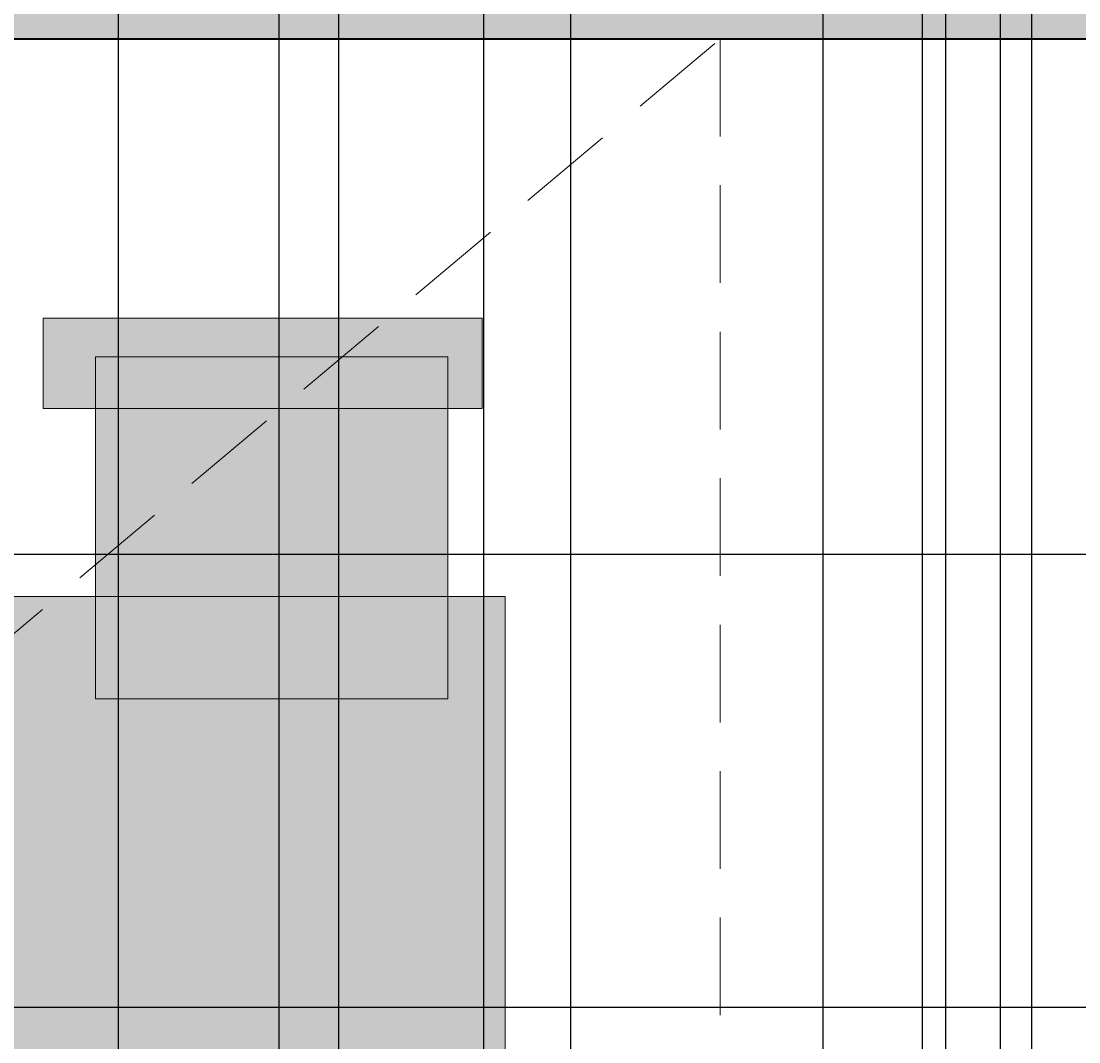
# Model space of a CAD drawing. Units: inches. Extents: x 818 to 1898, y 976 to 2364.
# Tile 76 of 96: x 1372 to 1439, y 1980 to 2045. Entities that reach past the tile are written whole.
import ezdxf

# ---------------------------------------------------------------- set-up
doc = ezdxf.new("R2010")
doc.units = ezdxf.units.IN
doc.header["$LTSCALE"] = 5
doc.header["$MEASUREMENT"] = 0
doc.linetypes.add('HIDDEN', pattern=[0.375, 0.25, -0.125])
for name, color, linetype, lineweight in [('A-ANNO-DIMS', 2, 'Continuous', 18), ('A-FLOR-OVHD', 8, 'HIDDEN', 13), ('A-FURN', 8, 'Continuous', 18), ('A-FURN-PATT', 8, 'Continuous', 9), ('A-GLAZ', 4, 'Continuous', 18), ('A-WALL', 7, 'Continuous', 40)]:
    doc.layers.add(name, color=color, linetype=linetype, lineweight=lineweight)
doc.layers.add('A-GLAZ-PATT', color=141, linetype='Continuous', lineweight=9, true_color=0xadddf7)
doc.layers.add('A-WALL-PATT', color=251, linetype='Continuous', lineweight=13, true_color=0x636466)
doc.styles.get("Standard").update_dxf_attribs({"font": 'arial.ttf'})
doc.dimstyles.get("Standard").update_dxf_attribs({"dimtxt": 0.18, "dimasz": 0.18, "dimexe": 0.18, "dimexo": 0.0625, "dimgap": 0.09, "dimtad": 0, "dimtih": 1, "dimtoh": 1, "dimdec": 4, "dimzin": 0, "dimdsep": 46, "dimtxsty": 'Standard', "dimcen": 0.09, "dimadec": 0, "dimazin": 0, "dimtfac": 1, "dimtdec": 4, "dimtofl": 0, "dimtmove": 0, "dimatfit": 3, "dimfxl": 1, "dimtolj": 1, "dimtzin": 0, "dimarcsym": 0})

# ---------------------------------------------------------------- blocks, each defined once
blk = doc.blocks.new('*D61')
at = {"layer": 'A-ANNO-DIMS', "color": 0, "lineweight": -2, "ltscale": 5, "transparency": 16777216}
for p, q in [((1071.725, 1203.027), (1071.725, 2363.873)), ((1071.905, 2363.693), (1250.936, 2363.693)), ((1430.545, 2363.693), (1251.514, 2363.693)), ((1430.725, 1203.027), (1430.725, 2363.873))]:
    blk.add_line(p, q, dxfattribs=at)
at = {"layer": 'A-ANNO-DIMS', "color": 0, "ltscale": 5, "transparency": 16777216}
for points in [[(1071.905, 2363.723), (1071.905, 2363.663), (1071.725, 2363.693)], [(1430.545, 2363.723), (1430.545, 2363.663), (1430.725, 2363.693)]]:
    blk.add_solid(points, dxfattribs=at)
at = {"layer": 'Defpoints', "color": 0, "ltscale": 5, "transparency": 16777216}
for p in [(1430.725, 2363.693), (1071.725, 1202.964), (1430.725, 1202.964)]:
    blk.add_point(p, dxfattribs=at)
at = {"layer": 'A-ANNO-DIMS', "color": 0, "ltscale": 5, "transparency": 16777216, "insert": (1251.225, 2363.693), "char_height": 0.18, "attachment_point": 5}
blk.add_mtext('\\A1;359', dxfattribs=at)
blk = doc.blocks.new('*D64')
at = {"layer": 'A-ANNO-DIMS', "color": 0, "lineweight": -2, "ltscale": 5, "transparency": 16777216}
for p, q in [((1197.725, 1501.141), (1197.725, 2363.873)), ((1197.905, 2363.693), (1313.935, 2363.693)), ((1430.545, 2363.693), (1314.516, 2363.693)), ((1430.725, 1501.141), (1430.725, 2363.873))]:
    blk.add_line(p, q, dxfattribs=at)
at = {"layer": 'A-ANNO-DIMS', "color": 0, "ltscale": 5, "transparency": 16777216}
for points in [[(1197.905, 2363.723), (1197.905, 2363.663), (1197.725, 2363.693)], [(1430.545, 2363.723), (1430.545, 2363.663), (1430.725, 2363.693)]]:
    blk.add_solid(points, dxfattribs=at)
at = {"layer": 'Defpoints', "color": 0, "ltscale": 5, "transparency": 16777216}
for p in [(1430.725, 2363.693), (1197.725, 1501.078), (1430.725, 1501.078)]:
    blk.add_point(p, dxfattribs=at)
at = {"layer": 'A-ANNO-DIMS', "color": 0, "ltscale": 5, "transparency": 16777216, "insert": (1314.225, 2363.693), "char_height": 0.18, "attachment_point": 5}
blk.add_mtext('\\A1;233', dxfattribs=at)
blk = doc.blocks.new('*D73')
at = {"layer": 'A-ANNO-DIMS', "color": 0, "lineweight": -2, "ltscale": 5, "transparency": 16777216}
for p, q in [((1590.663, 2011.078), (818.026, 2011.078)), ((818.206, 2010.898), (818.206, 1996.76)), ((818.206, 1982.258), (818.206, 1996.396)), ((1590.663, 1982.078), (818.026, 1982.078))]:
    blk.add_line(p, q, dxfattribs=at)
at = {"layer": 'A-ANNO-DIMS', "color": 0, "ltscale": 5, "transparency": 16777216}
for points in [[(818.176, 2010.898), (818.236, 2010.898), (818.206, 2011.078)], [(818.176, 1982.258), (818.236, 1982.258), (818.206, 1982.078)]]:
    blk.add_solid(points, dxfattribs=at)
at = {"layer": 'Defpoints', "color": 0, "ltscale": 5, "transparency": 16777216}
for p in [(818.206, 2011.078), (1590.725, 2011.078), (1590.725, 1982.078)]:
    blk.add_point(p, dxfattribs=at)
at = {"layer": 'A-ANNO-DIMS', "color": 0, "ltscale": 5, "transparency": 16777216, "insert": (818.206, 1996.578), "char_height": 0.18, "attachment_point": 5}
blk.add_mtext('\\A1;29', dxfattribs=at)
blk = doc.blocks.new('*D85')
at = {"layer": 'A-ANNO-DIMS', "color": 0, "lineweight": -2, "ltscale": 5, "transparency": 16777216}
for p, q in [((1258.788, 2053.078), (1897.916, 2053.078)), ((1897.736, 2052.898), (1897.736, 1876.76)), ((1897.736, 1700.258), (1897.736, 1876.396)), ((1258.788, 1700.078), (1897.916, 1700.078))]:
    blk.add_line(p, q, dxfattribs=at)
at = {"layer": 'A-ANNO-DIMS', "color": 0, "ltscale": 5, "transparency": 16777216}
for points in [[(1897.706, 2052.898), (1897.766, 2052.898), (1897.736, 2053.078)], [(1897.706, 1700.258), (1897.766, 1700.258), (1897.736, 1700.078)]]:
    blk.add_solid(points, dxfattribs=at)
at = {"layer": 'Defpoints', "color": 0, "ltscale": 5, "transparency": 16777216}
for p in [(1258.725, 2053.078), (1897.736, 2053.078), (1258.725, 1700.078)]:
    blk.add_point(p, dxfattribs=at)
at = {"layer": 'A-ANNO-DIMS', "color": 0, "ltscale": 5, "transparency": 16777216, "insert": (1897.736, 1876.578), "char_height": 0.18, "attachment_point": 5}
blk.add_mtext('\\A1;353', dxfattribs=at)
blk = doc.blocks.new('*D98')
at = {"layer": 'A-ANNO-DIMS', "color": 0, "lineweight": -2, "ltscale": 5, "transparency": 16777216}
for p, q in [((1338.541, 1071.118), (1338.541, 2363.873)), ((1338.721, 2363.693), (1364.815, 2363.693)), ((1391.696, 2363.693), (1365.602, 2363.693)), ((1391.876, 1071.118), (1391.876, 2363.873))]:
    blk.add_line(p, q, dxfattribs=at)
at = {"layer": 'A-ANNO-DIMS', "color": 0, "ltscale": 5, "transparency": 16777216}
for points in [[(1338.721, 2363.723), (1338.721, 2363.663), (1338.541, 2363.693)], [(1391.696, 2363.723), (1391.696, 2363.663), (1391.876, 2363.693)]]:
    blk.add_solid(points, dxfattribs=at)
at = {"layer": 'Defpoints', "color": 0, "ltscale": 5, "transparency": 16777216}
for p in [(1391.876, 2363.693), (1338.541, 1071.055), (1391.876, 1071.055)]:
    blk.add_point(p, dxfattribs=at)
at = {"layer": 'A-ANNO-DIMS', "color": 0, "ltscale": 5, "transparency": 16777216, "insert": (1365.208, 2363.693), "char_height": 0.18, "attachment_point": 5}
blk.add_mtext('\\A1;53.33', dxfattribs=at)
blk = doc.blocks.new('*D99')
at = {"layer": 'A-ANNO-DIMS', "color": 0, "lineweight": -2, "ltscale": 5, "transparency": 16777216}
for p, q in [((1391.876, 1071.118), (1391.876, 2363.873)), ((1392.056, 2363.693), (1420.454, 2363.693)), ((1449.64, 2363.693), (1421.241, 2363.693)), ((1449.82, 1071.118), (1449.82, 2363.873))]:
    blk.add_line(p, q, dxfattribs=at)
at = {"layer": 'A-ANNO-DIMS', "color": 0, "ltscale": 5, "transparency": 16777216}
for points in [[(1392.056, 2363.723), (1392.056, 2363.663), (1391.876, 2363.693)], [(1449.64, 2363.723), (1449.64, 2363.663), (1449.82, 2363.693)]]:
    blk.add_solid(points, dxfattribs=at)
at = {"layer": 'Defpoints', "color": 0, "ltscale": 5, "transparency": 16777216}
for p in [(1449.82, 2363.693), (1391.876, 1071.055), (1449.82, 1071.055)]:
    blk.add_point(p, dxfattribs=at)
at = {"layer": 'A-ANNO-DIMS', "color": 0, "ltscale": 5, "transparency": 16777216, "insert": (1420.848, 2363.693), "char_height": 0.18, "attachment_point": 5}
blk.add_mtext('\\A1;57.94', dxfattribs=at)
blk = doc.blocks.new('*D161')
at = {"layer": 'A-ANNO-DIMS', "color": 0, "lineweight": -2, "ltscale": 5, "transparency": 16777216}
for p, q in [((1429.225, 1876.141), (1429.225, 2363.873)), ((1429.405, 2363.693), (1509.589, 2363.693)), ((1590.545, 2363.693), (1510.361, 2363.693)), ((1590.725, 1876.141), (1590.725, 2363.873))]:
    blk.add_line(p, q, dxfattribs=at)
at = {"layer": 'A-ANNO-DIMS', "color": 0, "ltscale": 5, "transparency": 16777216}
for points in [[(1429.405, 2363.723), (1429.405, 2363.663), (1429.225, 2363.693)], [(1590.545, 2363.723), (1590.545, 2363.663), (1590.725, 2363.693)]]:
    blk.add_solid(points, dxfattribs=at)
at = {"layer": 'Defpoints', "color": 0, "ltscale": 5, "transparency": 16777216}
for p in [(1590.725, 2363.693), (1429.225, 1876.078), (1590.725, 1876.078)]:
    blk.add_point(p, dxfattribs=at)
at = {"layer": 'A-ANNO-DIMS', "color": 0, "ltscale": 5, "transparency": 16777216, "insert": (1509.975, 2363.693), "char_height": 0.18, "attachment_point": 5}
blk.add_mtext('\\A1;161.5', dxfattribs=at)
blk = doc.blocks.new('*D166')
at = {"layer": 'A-ANNO-DIMS', "color": 0, "lineweight": -2, "ltscale": 5, "transparency": 16777216}
for p, q in [((1401.146, 1510.141), (1401.146, 2363.873)), ((1401.326, 2363.693), (1415.54, 2363.693)), ((1430.545, 2363.693), (1416.331, 2363.693)), ((1430.725, 1510.141), (1430.725, 2363.873))]:
    blk.add_line(p, q, dxfattribs=at)
at = {"layer": 'A-ANNO-DIMS', "color": 0, "ltscale": 5, "transparency": 16777216}
for points in [[(1401.326, 2363.723), (1401.326, 2363.663), (1401.146, 2363.693)], [(1430.545, 2363.723), (1430.545, 2363.663), (1430.725, 2363.693)]]:
    blk.add_solid(points, dxfattribs=at)
at = {"layer": 'Defpoints', "color": 0, "ltscale": 5, "transparency": 16777216}
for p in [(1430.725, 2363.693), (1401.146, 1510.078), (1430.725, 1510.078)]:
    blk.add_point(p, dxfattribs=at)
at = {"layer": 'A-ANNO-DIMS', "color": 0, "ltscale": 5, "transparency": 16777216, "insert": (1415.936, 2363.693), "char_height": 0.18, "attachment_point": 5}
blk.add_mtext('\\A1;29.58', dxfattribs=at)
blk = doc.blocks.new('*D191')
at = {"layer": 'A-ANNO-DIMS', "color": 0, "lineweight": -2, "ltscale": 5, "transparency": 16777216}
for p, q in [((1434.225, 1409.115), (1434.225, 2363.873)), ((1434.405, 2363.693), (1435.076, 2363.693)), ((1436.045, 2363.693), (1435.375, 2363.693)), ((1436.225, 1409.115), (1436.225, 2363.873))]:
    blk.add_line(p, q, dxfattribs=at)
at = {"layer": 'A-ANNO-DIMS', "color": 0, "ltscale": 5, "transparency": 16777216}
for points in [[(1434.405, 2363.723), (1434.405, 2363.663), (1434.225, 2363.693)], [(1436.045, 2363.723), (1436.045, 2363.663), (1436.225, 2363.693)]]:
    blk.add_solid(points, dxfattribs=at)
at = {"layer": 'Defpoints', "color": 0, "ltscale": 5, "transparency": 16777216}
for p in [(1436.225, 2363.693), (1434.225, 1409.052), (1436.225, 1409.052)]:
    blk.add_point(p, dxfattribs=at)
at = {"layer": 'A-ANNO-DIMS', "color": 0, "ltscale": 5, "transparency": 16777216, "insert": (1435.225, 2363.693), "char_height": 0.18, "attachment_point": 5}
blk.add_mtext('\\A1;2', dxfattribs=at)
blk = doc.blocks.new('*D207')
at = {"layer": 'A-ANNO-DIMS', "color": 0, "lineweight": -2, "ltscale": 5, "transparency": 16777216}
for p, q in [((1590.663, 2044.078), (818.026, 2044.078)), ((818.206, 2043.898), (818.206, 2027.76)), ((818.206, 2011.258), (818.206, 2027.396)), ((1590.663, 2011.078), (818.026, 2011.078))]:
    blk.add_line(p, q, dxfattribs=at)
at = {"layer": 'A-ANNO-DIMS', "color": 0, "ltscale": 5, "transparency": 16777216}
for points in [[(818.176, 2043.898), (818.236, 2043.898), (818.206, 2044.078)], [(818.176, 2011.258), (818.236, 2011.258), (818.206, 2011.078)]]:
    blk.add_solid(points, dxfattribs=at)
at = {"layer": 'Defpoints', "color": 0, "ltscale": 5, "transparency": 16777216}
for p in [(818.206, 2044.078), (1590.725, 2044.078), (1590.725, 2011.078)]:
    blk.add_point(p, dxfattribs=at)
at = {"layer": 'A-ANNO-DIMS', "color": 0, "ltscale": 5, "transparency": 16777216, "insert": (818.206, 2027.578), "char_height": 0.18, "attachment_point": 5}
blk.add_mtext('\\A1;33', dxfattribs=at)
blk = doc.blocks.new('*D252')
at = {"layer": 'A-ANNO-DIMS', "color": 0, "lineweight": -2, "ltscale": 5, "transparency": 16777216}
for p, q in [((1330.305, 2053.016), (1330.305, 975.663)), ((1388.031, 2053.016), (1388.031, 975.663)), ((1330.485, 975.843), (1358.775, 975.843)), ((1387.851, 975.843), (1359.562, 975.843))]:
    blk.add_line(p, q, dxfattribs=at)
at = {"layer": 'A-ANNO-DIMS', "color": 0, "ltscale": 5, "transparency": 16777216}
for points in [[(1330.485, 975.873), (1330.485, 975.813), (1330.305, 975.843)], [(1387.851, 975.873), (1387.851, 975.813), (1388.031, 975.843)]]:
    blk.add_solid(points, dxfattribs=at)
at = {"layer": 'Defpoints', "color": 0, "ltscale": 5, "transparency": 16777216}
for p in [(1330.305, 2053.078), (1388.031, 2053.078), (1388.031, 975.843)]:
    blk.add_point(p, dxfattribs=at)
at = {"layer": 'A-ANNO-DIMS', "color": 0, "ltscale": 5, "transparency": 16777216, "insert": (1359.168, 975.843), "char_height": 0.18, "attachment_point": 5}
blk.add_mtext('\\A1;57.73', dxfattribs=at)
blk = doc.blocks.new('*D273')
at = {"layer": 'A-ANNO-DIMS', "color": 0, "lineweight": -2, "ltscale": 5, "transparency": 16777216}
for p, q in [((1406.725, 1587.479), (1406.725, 2363.873)), ((1406.905, 2363.693), (1418.505, 2363.693)), ((1430.545, 2363.693), (1418.945, 2363.693)), ((1430.725, 1587.479), (1430.725, 2363.873))]:
    blk.add_line(p, q, dxfattribs=at)
at = {"layer": 'A-ANNO-DIMS', "color": 0, "ltscale": 5, "transparency": 16777216}
for points in [[(1406.905, 2363.723), (1406.905, 2363.663), (1406.725, 2363.693)], [(1430.545, 2363.723), (1430.545, 2363.663), (1430.725, 2363.693)]]:
    blk.add_solid(points, dxfattribs=at)
at = {"layer": 'Defpoints', "color": 0, "ltscale": 5, "transparency": 16777216}
for p in [(1430.725, 2363.693), (1406.725, 1587.416), (1430.725, 1587.416)]:
    blk.add_point(p, dxfattribs=at)
at = {"layer": 'A-ANNO-DIMS', "color": 0, "ltscale": 5, "transparency": 16777216, "insert": (1418.725, 2363.693), "char_height": 0.18, "attachment_point": 5}
blk.add_mtext('\\A1;24', dxfattribs=at)
blk = doc.blocks.new('*D274')
at = {"layer": 'A-ANNO-DIMS', "color": 0, "lineweight": -2, "ltscale": 5, "transparency": 16777216}
for p, q in [((1311.025, 1897.929), (1311.025, 2363.873)), ((1311.205, 2363.693), (1344.007, 2363.693)), ((1377.599, 2363.693), (1344.797, 2363.693)), ((1377.779, 1897.929), (1377.779, 2363.873))]:
    blk.add_line(p, q, dxfattribs=at)
at = {"layer": 'A-ANNO-DIMS', "color": 0, "ltscale": 5, "transparency": 16777216}
for points in [[(1311.205, 2363.723), (1311.205, 2363.663), (1311.025, 2363.693)], [(1377.599, 2363.723), (1377.599, 2363.663), (1377.779, 2363.693)]]:
    blk.add_solid(points, dxfattribs=at)
at = {"layer": 'Defpoints', "color": 0, "ltscale": 5, "transparency": 16777216}
for p in [(1377.779, 2363.693), (1311.025, 1897.866), (1377.779, 1897.866)]:
    blk.add_point(p, dxfattribs=at)
at = {"layer": 'A-ANNO-DIMS', "color": 0, "ltscale": 5, "transparency": 16777216, "insert": (1344.402, 2363.693), "char_height": 0.18, "attachment_point": 5}
blk.add_mtext('\\A1;66.75', dxfattribs=at)
blk = doc.blocks.new('*D281')
at = {"layer": 'A-ANNO-DIMS', "color": 0, "lineweight": -2, "ltscale": 5, "transparency": 16777216}
for p, q in [((1250.303, 1913.703), (1250.303, 2363.873)), ((1250.483, 2363.693), (1420.121, 2363.693)), ((1590.545, 2363.693), (1420.907, 2363.693)), ((1590.725, 2011.141), (1590.725, 2363.873))]:
    blk.add_line(p, q, dxfattribs=at)
at = {"layer": 'A-ANNO-DIMS', "color": 0, "ltscale": 5, "transparency": 16777216}
for points in [[(1250.483, 2363.723), (1250.483, 2363.663), (1250.303, 2363.693)], [(1590.545, 2363.723), (1590.545, 2363.663), (1590.725, 2363.693)]]:
    blk.add_solid(points, dxfattribs=at)
at = {"layer": 'Defpoints', "color": 0, "ltscale": 5, "transparency": 16777216}
for p in [(1590.725, 2363.693), (1590.725, 2011.078), (1250.303, 1913.64)]:
    blk.add_point(p, dxfattribs=at)
at = {"layer": 'A-ANNO-DIMS', "color": 0, "ltscale": 5, "transparency": 16777216, "insert": (1420.514, 2363.693), "char_height": 0.18, "attachment_point": 5}
blk.add_mtext('\\A1;340.4', dxfattribs=at)
blk = doc.blocks.new('*D282')
at = {"layer": 'A-ANNO-DIMS', "color": 0, "lineweight": -2, "ltscale": 5, "transparency": 16777216}
for p, q in [((1422.083, 2081.188), (1897.916, 2081.188)), ((1897.736, 2081.008), (1897.736, 1884.315)), ((1897.736, 1687.258), (1897.736, 1883.951)), ((1463.788, 1687.078), (1897.916, 1687.078))]:
    blk.add_line(p, q, dxfattribs=at)
at = {"layer": 'A-ANNO-DIMS', "color": 0, "ltscale": 5, "transparency": 16777216}
for points in [[(1897.706, 2081.008), (1897.766, 2081.008), (1897.736, 2081.188)], [(1897.706, 1687.258), (1897.766, 1687.258), (1897.736, 1687.078)]]:
    blk.add_solid(points, dxfattribs=at)
at = {"layer": 'Defpoints', "color": 0, "ltscale": 5, "transparency": 16777216}
for p in [(1422.02, 2081.188), (1897.736, 2081.188), (1463.725, 1687.078)]:
    blk.add_point(p, dxfattribs=at)
at = {"layer": 'A-ANNO-DIMS', "color": 0, "ltscale": 5, "transparency": 16777216, "insert": (1897.736, 1884.133), "char_height": 0.18, "attachment_point": 5}
blk.add_mtext('\\A1;394.1', dxfattribs=at)
blk = doc.blocks.new('*D288')
at = {"layer": 'A-ANNO-DIMS', "color": 0, "lineweight": -2, "ltscale": 5, "transparency": 16777216}
for p, q in [((1422.876, 1742.674), (1422.876, 2363.873)), ((1423.056, 2363.693), (1466.906, 2363.693)), ((1511.545, 2363.693), (1467.695, 2363.693)), ((1511.725, 1716.108), (1511.725, 2363.873))]:
    blk.add_line(p, q, dxfattribs=at)
at = {"layer": 'A-ANNO-DIMS', "color": 0, "ltscale": 5, "transparency": 16777216}
for points in [[(1423.056, 2363.723), (1423.056, 2363.663), (1422.876, 2363.693)], [(1511.545, 2363.723), (1511.545, 2363.663), (1511.725, 2363.693)]]:
    blk.add_solid(points, dxfattribs=at)
at = {"layer": 'Defpoints', "color": 0, "ltscale": 5, "transparency": 16777216}
for p in [(1511.725, 2363.693), (1422.876, 1742.611), (1511.725, 1716.045)]:
    blk.add_point(p, dxfattribs=at)
at = {"layer": 'A-ANNO-DIMS', "color": 0, "ltscale": 5, "transparency": 16777216, "insert": (1467.3, 2363.693), "char_height": 0.18, "attachment_point": 5}
blk.add_mtext('\\A1;88.85', dxfattribs=at)

msp = doc.modelspace()

# ---------------------------------------------------------------- hatches: boundary and pattern name
at = {"layer": 'A-FURN-PATT', "ltscale": 5}
h = msp.add_hatch(color=256, dxfattribs=at)
h.dxf.hatch_style = 1
h.paths.add_polyline_path([(1341.9997, 1981.5338), (1317.9034, 2001.8247), (1314.2595, 2001.8247), (1314.2595, 2004.893), (1310.1046, 2008.3917), (1303.9314, 2008.3917), (1303.9314, 1953.0408), (1308.1629, 1953.0408), (1314.2595, 1958.1746), (1314.2595, 1959.6079), (1315.9616, 1959.6079)])
h.paths.add_polyline_path([(1341.9997, 1981.5338), (1315.9616, 1959.6079), (1336.7936, 1959.6079), (1336.7936, 1953.0408), (1345.3966, 1953.0408), (1345.3966, 1959.6079), (1368.0379, 1959.6079)])
h.paths.add_polyline_path([(1402.518, 2008.3917), (1398.8475, 2008.3917), (1398.8475, 2001.8247), (1376.3134, 2001.8247), (1376.3134, 2008.3917), (1373.8948, 2008.3917), (1367.9307, 2003.3695), (1367.9307, 2001.8247), (1366.0961, 2001.8247), (1341.9997, 1981.5338), (1368.0379, 1959.6079), (1375.8366, 1953.0408), (1376.3134, 1953.0408), (1376.3134, 1959.6079), (1398.8475, 1959.6079), (1398.8475, 1953.0408), (1402.518, 1953.0408)])
h.paths.add_polyline_path([(1366.0961, 2001.8247), (1345.3966, 2001.8247), (1345.3966, 2008.3917), (1336.7936, 2008.3917), (1336.7936, 2001.8247), (1317.9034, 2001.8247), (1341.9997, 1981.5338)])
h.paths.add_polyline_path([(1336.7936, 1959.6079), (1315.9616, 1959.6079), (1314.2595, 1958.1746), (1314.2595, 1953.0408), (1336.7936, 1953.0408)], flags=17)
h.paths.add_polyline_path([(1367.9307, 1959.6079), (1345.3966, 1959.6079), (1345.3966, 1953.0408), (1367.9307, 1953.0408)], flags=17)
h.paths.add_polyline_path([(1398.8475, 1959.6079), (1376.3134, 1959.6079), (1376.3134, 1953.0408), (1398.8475, 1953.0408)], flags=17)
h.paths.add_polyline_path([(1368.0379, 1959.6079), (1367.9307, 1959.6079), (1367.9307, 1953.0408), (1375.8366, 1953.0408)], flags=17)
h.paths.add_polyline_path([(1314.2595, 1958.1746), (1308.1629, 1953.0408), (1314.2595, 1953.0408)], flags=17)
h.paths.add_polyline_path([(1315.9616, 1959.6079), (1314.2595, 1959.6079), (1314.2595, 1958.1746)], flags=16)
h.paths.add_polyline_path([(1314.2595, 2008.3917), (1310.1046, 2008.3917), (1314.2595, 2004.893)], flags=17)
h.paths.add_polyline_path([(1336.7936, 2008.3917), (1314.2595, 2008.3917), (1314.2595, 2004.893), (1317.9034, 2001.8247), (1336.7936, 2001.8247)], flags=17)
h.paths.add_polyline_path([(1314.2595, 2004.893), (1314.2595, 2001.8247), (1317.9034, 2001.8247)], flags=16)
h.paths.add_polyline_path([(1367.9307, 2008.3917), (1345.3966, 2008.3917), (1345.3966, 2001.8247), (1366.0961, 2001.8247), (1367.9307, 2003.3695)], flags=17)
h.paths.add_polyline_path([(1398.8475, 2008.3917), (1376.3134, 2008.3917), (1376.3134, 2001.8247), (1398.8475, 2001.8247)], flags=17)
h.paths.add_polyline_path([(1373.8948, 2008.3917), (1367.9307, 2008.3917), (1367.9307, 2003.3695)], flags=17)
h.paths.add_polyline_path([(1367.9307, 2003.3695), (1366.0961, 2001.8247), (1367.9307, 2001.8247)], flags=16)
h.paths.add_polyline_path([(1546.1595, 2044.0782), (1451.7698, 2044.0782), (1451.7698, 2020.0782), (1546.1595, 2020.0782)])
h.paths.add_polyline_path([(1492.0729, 2040.001, 0.431429), (1491.8238, 2040.251), (1491.3087, 2040.251, 0.415217), (1491.0729, 2040.001)], flags=16)
h.paths.add_polyline_path([(1481.8346, 2039.6036), (1511.886, 2039.6036), (1511.886, 2024.9917), (1481.8346, 2024.9917)], flags=16)
h.paths.add_polyline_path([(1491.0729, 2039.4857), (1491.0729, 2039.501), (1492.0729, 2039.501, -0.4117484), (1491.8401, 2039.251), (1491.8229, 2039.251), (1491.8229, 2039.2509, 0.4325918), (1492.0729, 2039.501), (1491.0729, 2039.501, 0.432604), (1491.3229, 2039.2509), (1491.3229, 2039.251), (1491.325, 2039.251, -0.4165823)], flags=0)
h.paths.add_polyline_path([(1485.3701, 2030.9622), (1485.3701, 2034.3556, -0.4142136), (1488.3701, 2037.3556), (1490.3421, 2037.3556, -0.0779193), (1491.0729, 2038.751), (1495.0729, 2038.751, -0.3148679), (1496.07, 2037.1201, -0.3016609), (1497.9049, 2034.3556), (1497.9049, 2030.9622, -0.4142136), (1494.9049, 2027.9622), (1488.3701, 2027.9622, -0.4142136)], flags=0)
h.paths.add_polyline_path([(1490.3229, 2035.751, 0.2655648), (1491.3229, 2036.751), (1491.3229, 2037.126), (1491.0729, 2037.126, -0.7914183), (1490.5434, 2037.251, -0.7914183), (1491.0729, 2037.376), (1491.3229, 2037.376), (1491.3229, 2037.751), (1492.0729, 2037.751), (1492.0729, 2037.376), (1492.3229, 2037.376, -0.7914183), (1492.8524, 2037.251, -0.7914183), (1492.3229, 2037.126), (1492.1491, 2037.126, -0.0866263), (1492.5376, 2036.0294, 0.1070481), (1493.0729, 2035.751), (1490.3229, 2035.751)], flags=0)
h.paths.add_polyline_path([(1491.9774, 2037.251, -1), (1491.4184, 2037.251, -1)], flags=0)
h.paths.add_polyline_path([(1500.0743, 2028.6045), (1500.0743, 2029.4074), (1510.8414, 2029.4074), (1510.8414, 2028.6045)], flags=0)
h.paths.add_polyline_path([(1500.0743, 2030.5314), (1500.0743, 2031.3342), (1510.8414, 2031.3342), (1510.8414, 2030.5314)], flags=0)
h.paths.add_polyline_path([(1500.0743, 2032.94), (1500.0743, 2033.7428), (1510.8414, 2033.7428), (1510.8414, 2032.94)], flags=0)
h.paths.add_polyline_path([(1500.0743, 2035.7499), (1500.0743, 2036.5528), (1510.8414, 2036.5528), (1510.8414, 2035.7499)], flags=0)
h.paths.add_polyline_path([(1590.7251, 2044.0782), (1576.1595, 2044.0782), (1576.1595, 2020.0782), (1590.7251, 2020.0782)])
h.paths.add_polyline_path([(1668.4429, 2044.0782), (1599.7252, 2044.0782), (1599.7252, 2020.0782), (1668.4429, 2020.0782)])
h.paths.add_polyline_path([(1621.2588, 2040.001, 0.431429), (1621.0097, 2040.251), (1620.4946, 2040.251, 0.415217), (1620.2588, 2040.001)], flags=16)
h.paths.add_polyline_path([(1611.0205, 2024.9917), (1611.0205, 2039.6036), (1641.0719, 2039.6036), (1641.0719, 2024.9917)], flags=16)
h.paths.add_polyline_path([(1620.2588, 2039.4857), (1620.2588, 2039.501), (1621.2588, 2039.501, -0.4117484), (1621.026, 2039.251), (1621.0088, 2039.251), (1621.0088, 2039.2509, 0.4325918), (1621.2588, 2039.501), (1620.2588, 2039.501, 0.432604), (1620.5088, 2039.2509), (1620.5088, 2039.251), (1620.5109, 2039.251, -0.4165823)], flags=0)
h.paths.add_polyline_path([(1614.556, 2030.9622), (1614.556, 2034.3556, -0.4142136), (1617.556, 2037.3556), (1619.528, 2037.3556, -0.0779193), (1620.2588, 2038.751), (1624.2588, 2038.751, -0.3148679), (1625.2559, 2037.1201, -0.3016609), (1627.0908, 2034.3556), (1627.0908, 2030.9622, -0.4142136), (1624.0908, 2027.9622), (1617.556, 2027.9622, -0.4142136)], flags=0)
h.paths.add_polyline_path([(1619.5088, 2035.751, 0.2655648), (1620.5088, 2036.751), (1620.5088, 2037.126), (1620.2588, 2037.126, -0.7914183), (1619.7293, 2037.251, -0.7914183), (1620.2588, 2037.376), (1620.5088, 2037.376), (1620.5088, 2037.751), (1621.2588, 2037.751), (1621.2588, 2037.376), (1621.5088, 2037.376, -0.7914183), (1622.0383, 2037.251, -0.7914183), (1621.5088, 2037.126), (1621.335, 2037.126, -0.0866263), (1621.7235, 2036.0294, 0.1070481), (1622.2588, 2035.751), (1619.5088, 2035.751)], flags=0)
h.paths.add_polyline_path([(1620.6043, 2037.251, -1), (1621.1633, 2037.251, -1)], flags=0)
h.paths.add_polyline_path([(1629.2602, 2028.6045), (1629.2602, 2029.4074), (1640.0273, 2029.4074), (1640.0273, 2028.6045)], flags=0)
h.paths.add_polyline_path([(1629.2602, 2030.5314), (1629.2602, 2031.3342), (1640.0273, 2031.3342), (1640.0273, 2030.5314)], flags=0)
h.paths.add_polyline_path([(1629.2602, 2032.94), (1629.2602, 2033.7428), (1640.0273, 2033.7428), (1640.0273, 2032.94)], flags=0)
h.paths.add_polyline_path([(1629.2602, 2035.7499), (1629.2602, 2036.5528), (1640.0273, 2036.5528), (1640.0273, 2035.7499)], flags=0)
h.paths.add_polyline_path([(1705.7252, 2044.0782), (1698.4429, 2044.0782), (1698.4429, 2020.0782), (1705.7252, 2020.0782)])
h.paths.add_polyline_path([(1705.7252, 1972.0782), (1599.7252, 1972.0782), (1599.7252, 1948.0782), (1705.7252, 1948.0782)])
h.paths.add_polyline_path([(1550.0109, 1979.2444), (1483.5451, 1979.2444), (1483.5451, 1948.6602), (1550.0109, 1948.6602)])
h.paths.add_polyline_path([(1490.2586, 1948.6602), (1488.2586, 1948.6602), (1488.2586, 1941.1742, 0.4142136), (1491.2586, 1938.1742), (1500.7446, 1938.1742, -0.4142136)])
h.paths.add_polyline_path([(1513.2306, 1941.1742), (1513.2306, 1948.6602), (1511.2306, 1948.6602, -0.4142136), (1500.7446, 1938.1742), (1510.2306, 1938.1742, 0.4142136)])
h.paths.add_polyline_path([(1518.778, 1948.6602), (1516.778, 1948.6602), (1516.778, 1941.1742, 0.4142136), (1519.778, 1938.1742), (1529.264, 1938.1742, -0.4142136)])
h.paths.add_polyline_path([(1541.75, 1941.1742), (1541.75, 1948.6602), (1539.75, 1948.6602, -0.4142136), (1529.264, 1938.1742), (1538.75, 1938.1742, 0.4142136)])
h.paths.add_polyline_path([(1590.7251, 1900.0782), (1519.6413, 1900.0782), (1519.6413, 1876.0782), (1590.7251, 1876.0782)])
h = msp.add_hatch(color=256, dxfattribs=at)
h.dxf.hatch_style = 1
h.paths.add_polyline_path([(1336.7936, 1953.0408), (1314.2595, 1953.0408), (1314.2595, 1941.0096), (1336.7936, 1941.0096)])
h.paths.add_polyline_path([(1338.9915, 1941.0096), (1336.7936, 1941.0096), (1336.7936, 1937.7177), (1314.2595, 1937.7177), (1314.2595, 1941.0096), (1310.9077, 1941.0096), (1310.9077, 1935.2252), (1338.9915, 1935.2252)])
h.paths.add_polyline_path([(1336.7936, 1941.0096), (1314.2595, 1941.0096), (1314.2595, 1937.7177), (1336.7936, 1937.7177)], flags=17)
h.paths.add_polyline_path([(1367.9307, 1959.6079), (1345.3966, 1959.6079), (1345.3966, 1941.0096), (1367.9307, 1941.0096)])
h.paths.add_polyline_path([(1398.8475, 1953.0408), (1376.3134, 1953.0408), (1376.3134, 1952.6393), (1390.1242, 1941.0096), (1398.8475, 1941.0096)])
h.paths.add_polyline_path([(1376.3134, 1952.6393), (1376.3134, 1941.0096), (1390.1242, 1941.0096)], flags=17)
h.paths.add_polyline_path([(1370.1286, 1941.0096), (1367.9307, 1941.0096), (1367.9307, 1937.7177), (1345.3966, 1937.7177), (1345.3966, 1941.0096), (1342.0448, 1941.0096), (1342.0448, 1935.2252), (1370.1286, 1935.2252)])
h.paths.add_polyline_path([(1367.9307, 1941.0096), (1345.3966, 1941.0096), (1345.3966, 1937.7177), (1367.9307, 1937.7177)], flags=17)
h.paths.add_polyline_path([(1390.1242, 1941.0096), (1376.3134, 1941.0096), (1376.3134, 1937.7177), (1394.0336, 1937.7177)], flags=17)
h.paths.add_polyline_path([(1394.0336, 1937.7177), (1376.3134, 1937.7177), (1376.3134, 1941.0096), (1372.9616, 1941.0096), (1372.9616, 1935.2252), (1396.9935, 1935.2252)])
h.paths.add_polyline_path([(1398.8475, 1941.0096), (1390.1242, 1941.0096), (1394.0336, 1937.7177), (1398.8475, 1937.7177)])
h.paths.add_polyline_path([(1401.0455, 1941.0096), (1398.8475, 1941.0096), (1398.8475, 1937.7177), (1394.0336, 1937.7177), (1396.9935, 1935.2252), (1401.0455, 1935.2252)])
h.paths.add_polyline_path([(1336.7936, 2020.4229), (1314.2595, 2020.4229), (1314.2595, 2008.3917), (1336.7936, 2008.3917)])
h.paths.add_polyline_path([(1336.7936, 2023.7149), (1314.2595, 2023.7149), (1314.2595, 2020.4229), (1336.7936, 2020.4229)], flags=17)
h.paths.add_polyline_path([(1338.9915, 2026.2074), (1310.9077, 2026.2074), (1310.9077, 2020.4229), (1314.2595, 2020.4229), (1314.2595, 2023.7149), (1336.7936, 2023.7149), (1336.7936, 2020.4229), (1338.9915, 2020.4229)])
h.paths.add_polyline_path([(1367.9307, 2023.7149), (1345.3966, 2023.7149), (1345.3966, 2020.4229), (1367.9307, 2020.4229)], flags=17)
h.paths.add_polyline_path([(1370.1286, 2026.2074), (1342.0448, 2026.2074), (1342.0448, 2020.4229), (1345.3966, 2020.4229), (1345.3966, 2023.7149), (1367.9307, 2023.7149), (1367.9307, 2020.4229), (1370.1286, 2020.4229)])
h.paths.add_polyline_path([(1367.9307, 2020.4229), (1345.3966, 2020.4229), (1345.3966, 2008.3917), (1367.9307, 2008.3917)])
h.paths.add_polyline_path([(1398.8475, 2020.4229), (1388.1824, 2020.4229), (1376.3134, 2010.4284), (1376.3134, 2008.3917), (1398.8475, 2008.3917)])
h.paths.add_polyline_path([(1392.0918, 2023.7149), (1376.3134, 2023.7149), (1376.3134, 2020.4229), (1388.1824, 2020.4229)], flags=17)
h.paths.add_polyline_path([(1388.1824, 2020.4229), (1376.3134, 2020.4229), (1376.3134, 2010.4284)], flags=17)
h.paths.add_polyline_path([(1395.0518, 2026.2074), (1372.9616, 2026.2074), (1372.9616, 2020.4229), (1376.3134, 2020.4229), (1376.3134, 2023.7149), (1392.0918, 2023.7149)])
h.paths.add_polyline_path([(1398.8475, 2023.7149), (1392.0918, 2023.7149), (1388.1824, 2020.4229), (1398.8475, 2020.4229)])
h.paths.add_polyline_path([(1401.0455, 2026.2074), (1395.0518, 2026.2074), (1392.0918, 2023.7149), (1398.8475, 2023.7149), (1398.8475, 2020.4229), (1401.0455, 2020.4229)])
h.paths.add_polyline_path([(1327.0339, 1897.8663), (1311.025, 1897.8663), (1311.025, 1876.0782), (1327.0339, 1876.0782)])
h.paths.add_polyline_path([(1377.7791, 1897.8663), (1359.9579, 1897.8663), (1359.9579, 1876.0782), (1377.7791, 1876.0782)])
h.paths.add_polyline_path([(1430.7251, 1541.0439), (1406.7251, 1541.0439), (1406.7251, 1525.9965), (1430.7251, 1525.9965)])
h.paths.add_polyline_path([(1430.7251, 1587.4164), (1406.7251, 1587.4164), (1406.7251, 1570.9187), (1430.7251, 1570.9187)])
at = {"layer": 'A-GLAZ-PATT', "ltscale": 5}
h = msp.add_hatch(color=256, dxfattribs=at)
h.dxf.hatch_style = 1
h.paths.add_polyline_path([(1283.8183, 1504.5782), (1206.7252, 1504.5782), (1206.7252, 1501.0782), (1283.8183, 1501.0782)])
h.paths.add_polyline_path([(1283.8183, 1510.0782), (1206.7252, 1510.0782), (1206.7252, 1506.5782), (1283.8183, 1506.5782)])
h.paths.add_polyline_path([(1490.9163, 1355.0782), (1439.7252, 1355.0782), (1439.7252, 1409.0522), (1436.2251, 1409.0522), (1436.2251, 1351.5782), (1490.9163, 1351.5782)])
h.paths.add_polyline_path([(1434.2251, 1409.0522), (1430.7251, 1409.0522), (1430.7251, 1346.0782), (1435.0799, 1346.0782), (1435.0731, 1346.1152), (1435.1501, 1346.0782), (1490.9163, 1346.0782), (1490.9163, 1349.5782), (1434.2251, 1349.5782)])
h.paths.add_polyline_path([(1714.7252, 1545.0782), (1711.2252, 1545.0782), (1711.2252, 1521.0782), (1714.7252, 1521.0782)])
h.paths.add_polyline_path([(1709.2252, 1545.0782), (1705.7252, 1545.0782), (1705.7252, 1521.0782), (1709.2252, 1521.0782)])
h.paths.add_polyline_path([(1714.7252, 1687.0782), (1711.2252, 1687.0782), (1711.2252, 1649.9029), (1714.7252, 1649.9029)])
h.paths.add_polyline_path([(1709.2252, 1687.0782), (1705.7252, 1687.0782), (1705.7252, 1649.9029), (1709.2252, 1649.9029)])
h.paths.add_polyline_path([(1709.2252, 1745.5584), (1705.7252, 1745.5584), (1705.7252, 1717.3178), (1709.2252, 1717.3178)])
h.paths.add_polyline_path([(1714.7252, 1745.5584), (1711.2252, 1745.5584), (1711.2252, 1717.3178), (1714.7252, 1717.3178)])
h.paths.add_polyline_path([(1714.7252, 2014.5114), (1711.2252, 2014.5114), (1711.2252, 1962.0338), (1714.7252, 1962.0338)])
h.paths.add_polyline_path([(1709.2252, 2014.5114), (1705.7252, 2014.5114), (1705.7252, 1962.0338), (1709.2252, 1962.0338)])
h.paths.add_polyline_path([(1538.5155, 2047.5782), (1485.1216, 2047.5782), (1485.1216, 2044.0782), (1538.5155, 2044.0782)])
h.paths.add_polyline_path([(1538.5155, 2053.0782), (1485.1216, 2053.0782), (1485.1216, 2049.5782), (1538.5155, 2049.5782)])
h.paths.add_polyline_path([(1388.0315, 2047.5782), (1330.305, 2047.5782), (1330.305, 2044.0782), (1388.0315, 2044.0782)])
h.paths.add_polyline_path([(1388.0315, 2053.0782), (1330.305, 2053.0782), (1330.305, 2049.5782), (1388.0315, 2049.5782)])
h.paths.add_polyline_path([(1262.2252, 2019.2871), (1258.7251, 2019.2871), (1258.7251, 1928.9218), (1262.2252, 1928.9218)])
h.paths.add_polyline_path([(1267.7252, 2019.2871), (1264.2252, 2019.2871), (1264.2252, 1928.9218), (1267.7252, 1928.9218)])
h.paths.add_polyline_path([(1262.2252, 1862.9652), (1258.7251, 1862.9652), (1258.7251, 1814.9652), (1262.2252, 1814.9652)])
h.paths.add_polyline_path([(1267.7252, 1862.9652), (1264.2252, 1862.9652), (1264.2252, 1814.9652), (1267.7252, 1814.9652)])
h.paths.add_polyline_path([(1262.2252, 1755.3321), (1258.7251, 1755.3321), (1258.7251, 1707.3321), (1262.2252, 1707.3321)])
h.paths.add_polyline_path([(1267.7252, 1755.3321), (1264.2252, 1755.3321), (1264.2252, 1707.3321), (1267.7252, 1707.3321)])
h.paths.add_polyline_path([(1251.9333, 1692.5782), (1206.7252, 1692.5782), (1206.7252, 1687.0782), (1251.9333, 1687.0782)])
h.paths.add_polyline_path([(1251.9333, 1700.0782), (1206.7252, 1700.0782), (1206.7252, 1694.5782), (1251.9333, 1694.5782)])
at = {"layer": 'A-WALL-PATT', "ltscale": 5}
h = msp.add_hatch(color=256, dxfattribs=at)
h.dxf.hatch_style = 1
h.paths.add_polyline_path([(1267.7252, 1928.9218), (1258.7251, 1928.9218), (1258.7251, 1913.6401), (1250.3029, 1913.6401), (1250.3029, 1878.3919), (1258.7251, 1878.3919), (1258.7251, 1862.9652), (1267.7252, 1862.9652)])
h.paths.add_polyline_path([(1267.7252, 1814.9652), (1258.7251, 1814.9652), (1258.7251, 1755.3321), (1267.7252, 1755.3321)])
h.paths.add_polyline_path([(1463.7251, 1696.0782), (1267.7252, 1696.0782), (1267.7252, 1707.3321), (1258.7251, 1707.3321), (1258.7251, 1700.0782), (1251.9333, 1700.0782), (1251.9333, 1687.0782), (1463.7251, 1687.0782)])
h.paths.add_polyline_path([(1714.7252, 1717.3178), (1705.7252, 1717.3178), (1705.7252, 1696.0782), (1599.7252, 1696.0782), (1599.7252, 1790.0782), (1705.7252, 1790.0782), (1705.7252, 1785.6125), (1714.7252, 1785.6125), (1714.7252, 1827.2125), (1705.7252, 1827.2125), (1705.7252, 1802.0782), (1599.7252, 1802.0782), (1599.7252, 1867.0782), (1705.7252, 1867.0782), (1705.7252, 1857.2125), (1714.7252, 1857.2125), (1714.7252, 1930.0316), (1741.8409, 1930.0316), (1741.8409, 1935.0316), (1714.7252, 1935.0316), (1714.7252, 1957.0338), (1741.8409, 1957.0338), (1741.8409, 1962.0338), (1714.7252, 1962.0338), (1705.7252, 1962.0338), (1705.7252, 1948.0782), (1599.7252, 1948.0782), (1599.7252, 1981.0782), (1590.7251, 1981.0782), (1590.7251, 1941.0782), (1620.7252, 1941.0782), (1705.7252, 1941.0782), (1705.7252, 1876.0782), (1599.7252, 1876.0782), (1599.7252, 1911.0782), (1590.7251, 1911.0782), (1590.7251, 1876.0782), (1429.2251, 1876.0782), (1429.2251, 1867.0782), (1511.7251, 1867.0782), (1528.593, 1867.0782), (1595.7252, 1867.0782), (1595.7252, 1773.0782), (1520.7252, 1773.0782), (1520.7252, 1837.5823), (1532.593, 1837.5823), (1532.593, 1867.0782), (1528.593, 1867.0782), (1528.593, 1841.5823), (1511.7251, 1841.5823), (1511.7251, 1744.9714), (1520.7252, 1744.9714), (1520.7252, 1761.0782), (1595.7252, 1761.0782), (1595.7252, 1696.0782), (1520.7252, 1696.0782), (1520.7252, 1716.0454), (1511.7251, 1716.0454), (1511.7251, 1696.0782), (1511.7251, 1687.0782), (1714.7252, 1687.0782)])
h.paths.add_polyline_path([(1714.7252, 2053.0782), (1714.7252, 2081.1881), (1709.7252, 2081.1881), (1709.7252, 2053.0782), (1681.6446, 2053.0782), (1681.6446, 2081.1881), (1676.6446, 2081.1881), (1676.6446, 2053.0782), (1538.5155, 2053.0782), (1538.5155, 2044.0782), (1590.7251, 2044.0782), (1590.7251, 2011.0782), (1599.7252, 2011.0782), (1599.7252, 2044.0782), (1705.7252, 2044.0782), (1705.7252, 2014.5114), (1714.7252, 2014.5114)])
h.paths.add_polyline_path([(1485.1216, 2053.0782), (1422.02, 2053.0782), (1422.02, 2081.1881), (1413.02, 2081.1881), (1413.02, 2053.0782), (1399.6356, 2053.0782), (1399.6356, 2081.1881), (1390.6356, 2081.1881), (1390.6356, 2053.0782), (1388.0315, 2053.0782), (1388.0315, 2044.0782), (1416.2743, 2044.0782), (1485.1216, 2044.0782)])
h.paths.add_polyline_path([(1330.305, 2053.0782), (1258.7251, 2053.0782), (1258.7251, 2019.2871), (1267.7252, 2019.2871), (1267.7252, 2044.0782), (1330.305, 2044.0782)])
h.paths.add_polyline_path([(1258.7251, 2053.0782), (1214.6577, 2053.0782), (1214.6577, 2044.0782), (1258.7251, 2044.0782)])
h.paths.add_polyline_path([(1214.6577, 2053.0782), (1180.349, 2053.0782), (1180.349, 2044.0782), (1214.6577, 2044.0782)])
h.paths.add_polyline_path([(1714.7252, 1639.5782), (1741.8409, 1639.5782), (1741.8409, 1643.5782), (1714.7252, 1643.5782), (1714.7252, 1649.9029), (1705.7252, 1649.9029), (1705.7252, 1600.0782), (1477.7252, 1600.0782), (1477.7252, 1591.0782), (1520.7252, 1591.0782), (1616.7252, 1591.0782), (1616.7252, 1416.6857), (1622.7252, 1416.6857), (1622.7252, 1463.0782), (1624.7252, 1463.0782), (1624.7252, 1467.0782), (1622.7252, 1467.0782), (1622.7252, 1591.0782), (1705.7252, 1591.0782), (1705.7252, 1545.0782), (1714.7252, 1545.0782), (1741.8409, 1545.0782), (1741.8409, 1549.0782), (1714.7252, 1549.0782), (1714.7252, 1593.9175), (1737.8409, 1593.9175), (1737.8409, 1597.9175), (1714.7252, 1597.9175)])
h.paths.add_polyline_path([(1674.9024, 2060.7419), (1714.7045, 2060.7419), (1714.7045, 2073.1061), (1674.9024, 2073.1061)], flags=25)
h.paths.add_polyline_path([(1394.5468, 2061.6618), (1422.2344, 2061.6618), (1422.2344, 2074.0261), (1394.5468, 2074.0261)], flags=24)

# ---------------------------------------------------------------- linework, layer by layer
at = {"layer": 'A-FLOR-OVHD', "ltscale": 5}
msp.add_line((1267.7252, 1918.9894), (1416.2743, 2044.0782), dxfattribs=at)
msp.add_lwpolyline([(1267.7252, 2044.0782), (1416.2743, 2044.0782), (1416.2743, 1918.9894), (1267.7252, 1918.9894)], close=True, dxfattribs=at)
at = {"layer": 'A-FURN'}
for points in [[(1372.9616, 2020.4229), (1401.0455, 2020.4229), (1401.0455, 2026.2074), (1372.9616, 2026.2074)], [(1376.3134, 2001.8247), (1398.8475, 2001.8247), (1398.8475, 2023.7149), (1376.3134, 2023.7149)], [(1303.9314, 2008.3917), (1402.518, 2008.3917), (1402.518, 1953.0408), (1303.9314, 1953.0408)]]:
    msp.add_lwpolyline(points, close=True, dxfattribs=at)
at = {"layer": 'A-GLAZ'}
msp.add_line((1388.0315, 2053.0782), (1388.0315, 2044.0782), dxfattribs=at)
at = {"layer": 'A-WALL'}
msp.add_line((1267.7252, 2044.0782), (1590.7251, 2044.0782), dxfattribs=at)

# ---------------------------------------------------------------- dimensions: what is measured, and where the dimension line sits
at = {"layer": 'A-ANNO-DIMS', "ltscale": 5}
for base, p1, p2, override, picture, middle in [((1430.7251, 2363.6929), (1071.7251, 1202.9642), (1430.7251, 1202.9642), {"dimdec": 0, "dimlfac": 1, "dimrnd": 0, "dimzin": 0, "dimdsep": 46, "dimlunit": 2}, '*D61', (1251.2251, 2363.6929)), ((1430.7251, 2363.6929), (1197.7251, 1501.0782), (1430.7251, 1501.0782), {"dimdec": 0, "dimlfac": 1, "dimrnd": 0, "dimzin": 0, "dimdsep": 46, "dimlunit": 2}, '*D64', (1314.2251, 2363.6929)), ((1590.7251, 2363.6929), (1250.3029, 1913.6401), (1590.7251, 2011.0782), {"dimdec": 1, "dimlfac": 1, "dimrnd": 0, "dimzin": 0, "dimdsep": 46, "dimlunit": 2}, '*D281', (1420.514, 2363.6929)), ((1377.7791, 2363.6929), (1311.025, 1897.8663), (1377.7791, 1897.8663), {"dimdec": 2, "dimlfac": 1, "dimrnd": 0, "dimzin": 0, "dimdsep": 46, "dimlunit": 2}, '*D274', (1344.4021, 2363.6929)), ((1391.8757, 2363.6929), (1338.5412, 1071.0552), (1391.8757, 1071.0552), {"dimdec": 2, "dimlfac": 1, "dimrnd": 0, "dimzin": 0, "dimdsep": 46, "dimlunit": 2}, '*D98', (1365.2084, 2363.6929)), ((1449.8196, 2363.6929), (1391.8757, 1071.0552), (1449.8196, 1071.0552), {"dimdec": 2, "dimlfac": 1, "dimrnd": 0, "dimzin": 0, "dimdsep": 46, "dimlunit": 2}, '*D99', (1420.8477, 2363.6929)), ((1430.7251, 2363.6929), (1401.1463, 1510.0782), (1430.7251, 1510.0782), {"dimdec": 2, "dimlfac": 1, "dimrnd": 0, "dimzin": 0, "dimdsep": 46, "dimlunit": 2}, '*D166', (1415.9357, 2363.6929)), ((1430.7251, 2363.6929), (1406.7251, 1587.4164), (1430.7251, 1587.4164), {"dimdec": 0, "dimlfac": 1, "dimrnd": 0, "dimzin": 0, "dimdsep": 46, "dimlunit": 2}, '*D273', (1418.7251, 2363.6929)), ((1511.7251, 2363.6929), (1422.8756, 1742.6113), (1511.7251, 1716.0454), {"dimdec": 2, "dimlfac": 1, "dimrnd": 0, "dimzin": 0, "dimdsep": 46, "dimlunit": 2}, '*D288', (1467.3004, 2363.6929)), ((1590.7251, 2363.6929), (1429.2251, 1876.0782), (1590.7251, 1876.0782), {"dimdec": 1, "dimlfac": 1, "dimrnd": 0, "dimzin": 0, "dimdsep": 46, "dimlunit": 2}, '*D161', (1509.9751, 2363.6929)), ((1436.2251, 2363.6929), (1434.2251, 1409.0522), (1436.2251, 1409.0522), {"dimdec": 0, "dimlfac": 1, "dimrnd": 0, "dimzin": 0, "dimdsep": 46, "dimlunit": 2}, '*D191', (1435.2251, 2363.6929)), ((1388.0315, 975.8433), (1330.305, 2053.0782), (1388.0315, 2053.0782), {"dimdec": 2, "dimlfac": 1, "dimrnd": 0, "dimzin": 0, "dimdsep": 46, "dimlunit": 2}, '*D252', (1359.1682, 975.8433))]:
    dim = msp.add_linear_dim(base=base, p1=p1, p2=p2, dimstyle='Standard', override=override, dxfattribs=at)
    dim.commit()
    dim.dimension.update_dxf_attribs({"geometry": picture, "text_midpoint": middle})
for base, p1, p2, override, picture, middle in [((1897.736, 2081.1881), (1463.7251, 1687.0782), (1422.02, 2081.1881), {"dimdec": 1, "dimlfac": 1, "dimrnd": 0, "dimzin": 0, "dimdsep": 46, "dimlunit": 2}, '*D282', (1897.736, 1884.1332)), ((1897.736, 2053.0782), (1258.7251, 1700.0782), (1258.7251, 2053.0782), {"dimdec": 0, "dimlfac": 1, "dimrnd": 0, "dimzin": 0, "dimdsep": 46, "dimlunit": 2}, '*D85', (1897.736, 1876.5782)), ((818.2059, 2044.0782), (1590.7251, 2011.0782), (1590.7251, 2044.0782), {"dimdec": 0, "dimlfac": 1, "dimrnd": 0, "dimzin": 0, "dimdsep": 46, "dimlunit": 2}, '*D207', (818.2059, 2027.5782)), ((818.2059, 2011.0782), (1590.7251, 1982.0782), (1590.7251, 2011.0782), {"dimdec": 0, "dimlfac": 1, "dimrnd": 0, "dimzin": 0, "dimdsep": 46, "dimlunit": 2}, '*D73', (818.2059, 1996.5782))]:
    dim = msp.add_linear_dim(base=base, p1=p1, p2=p2, angle=90, dimstyle='Standard', override=override, dxfattribs=at)
    dim.commit()
    dim.dimension.update_dxf_attribs({"geometry": picture, "text_midpoint": middle})

doc.saveas('drawing.dxf')
